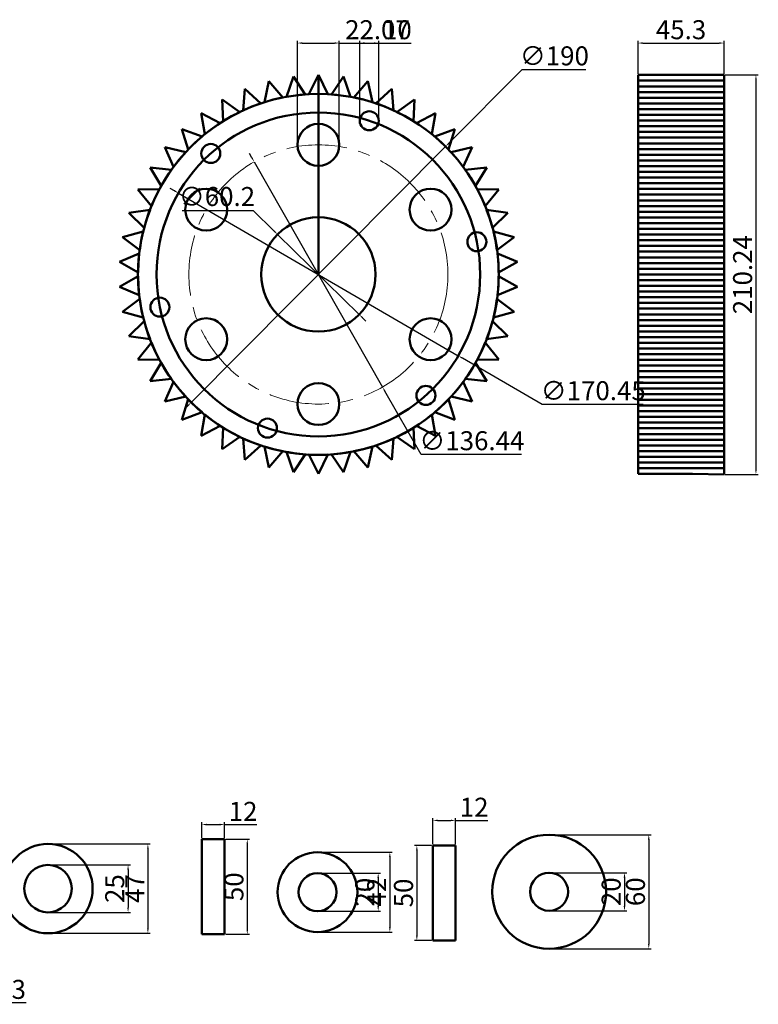
# Model space of a CAD drawing. Units: millimetres. Extents: x 828 to 2987, y 979 to 1807.
# Tile 4 of 6: x 1225 to 1614, y 1191 to 1709. Entities that reach past the tile are written whole.
import ezdxf

# ---------------------------------------------------------------- set-up
doc = ezdxf.new("R2010")
doc.units = ezdxf.units.MM
doc.linetypes.add('CENTER', pattern=[50.8, 31.75, -6.35, 6.35, -6.35])
for name, color, linetype, lineweight in [('M-CNTR', 1, 'CENTER', 18), ('M-DIMS', 2, 'Continuous', 25), ('M-OUTL', 7, 'Continuous', 50)]:
    doc.layers.add(name, color=color, linetype=linetype, lineweight=lineweight)
doc.styles.get("Standard").update_dxf_attribs({"font": 'arial.ttf'})
doc.dimstyles.new('ISO-25', dxfattribs={"dimtxt": 10, "dimasz": 2.5, "dimexe": 1.25, "dimexo": 0.625, "dimtad": 1, "dimtoh": 1, "dimdec": 0, "dimtxsty": 'Standard', "dimcen": 2.5, "dimadec": 0, "dimazin": 0, "dimtfac": 1, "dimtdec": 0, "dimtmove": 0, "dimatfit": 3, "dimfxl": 1, "dimarcsym": 0})

# ---------------------------------------------------------------- blocks, each defined once
blk = doc.blocks.new('*D29')
at = {"layer": 'Defpoints', "color": 0, "transparency": 16777216}
for p in [(1240.29, 1264.35), (1240.29, 1239.35), (1282.45, 1239.35)]:
    blk.add_point(p, dxfattribs=at)
at = {"layer": 'M-DIMS', "color": 0, "lineweight": -2, "transparency": 16777216}
for p, q in [((1240.91, 1264.35), (1283.7, 1264.35)), ((1282.45, 1261.85), (1282.45, 1241.85)), ((1240.91, 1239.35), (1283.7, 1239.35))]:
    blk.add_line(p, q, dxfattribs=at)
at = {"layer": 'M-DIMS', "color": 0, "transparency": 16777216}
for points in [[(1282.03, 1261.85), (1282.86, 1261.85), (1282.45, 1264.35)], [(1282.03, 1241.85), (1282.86, 1241.85), (1282.45, 1239.35)]]:
    blk.add_solid(points, dxfattribs=at)
at = {"layer": 'M-DIMS', "color": 0, "transparency": 16777216, "insert": (1276.72, 1251.85), "char_height": 10, "attachment_point": 5, "rotation": 90}
blk.add_mtext('25', dxfattribs=at)
blk = doc.blocks.new('*D30')
at = {"layer": 'Defpoints', "color": 0, "transparency": 16777216}
for p in [(1240.29, 1275.35), (1240.29, 1228.35), (1292.9, 1228.35)]:
    blk.add_point(p, dxfattribs=at)
at = {"layer": 'M-DIMS', "color": 0, "lineweight": -2, "transparency": 16777216}
for p, q in [((1240.91, 1275.35), (1294.15, 1275.35)), ((1292.9, 1272.85), (1292.9, 1230.85)), ((1240.91, 1228.35), (1294.15, 1228.35))]:
    blk.add_line(p, q, dxfattribs=at)
at = {"layer": 'M-DIMS', "color": 0, "transparency": 16777216}
for points in [[(1292.48, 1272.85), (1293.32, 1272.85), (1292.9, 1275.35)], [(1292.48, 1230.85), (1293.32, 1230.85), (1292.9, 1228.35)]]:
    blk.add_solid(points, dxfattribs=at)
at = {"layer": 'M-DIMS', "color": 0, "transparency": 16777216, "insert": (1287.28, 1251.85), "char_height": 10, "attachment_point": 5, "rotation": 90}
blk.add_mtext('47', dxfattribs=at)
blk = doc.blocks.new('*D31')
at = {"layer": 'Defpoints', "color": 0, "transparency": 16777216}
for p in [(1333.27, 1285.57), (1321.27, 1277.83), (1333.27, 1277.83)]:
    blk.add_point(p, dxfattribs=at)
at = {"layer": 'M-DIMS', "color": 0, "lineweight": -2, "transparency": 16777216}
for p, q in [((1321.27, 1278.45), (1321.27, 1286.82)), ((1323.77, 1285.57), (1330.77, 1285.57)), ((1333.27, 1278.45), (1333.27, 1286.82)), ((1333.27, 1285.57), (1350.3, 1285.57))]:
    blk.add_line(p, q, dxfattribs=at)
at = {"layer": 'M-DIMS', "color": 0, "transparency": 16777216}
for points in [[(1323.77, 1285.99), (1323.77, 1285.15), (1321.27, 1285.57)], [(1330.77, 1285.99), (1330.77, 1285.15), (1333.27, 1285.57)]]:
    blk.add_solid(points, dxfattribs=at)
at = {"layer": 'M-DIMS', "color": 0, "transparency": 16777216, "insert": (1343.03, 1291.22), "char_height": 10, "attachment_point": 5}
blk.add_mtext('12', dxfattribs=at)
blk = doc.blocks.new('*D32')
at = {"layer": 'Defpoints', "color": 0, "transparency": 16777216}
for p in [(1333.27, 1277.83), (1333.27, 1227.83), (1345.24, 1227.83)]:
    blk.add_point(p, dxfattribs=at)
at = {"layer": 'M-DIMS', "color": 0, "lineweight": -2, "transparency": 16777216}
for p, q in [((1333.89, 1277.83), (1346.49, 1277.83)), ((1345.24, 1275.33), (1345.24, 1230.33)), ((1333.89, 1227.83), (1346.49, 1227.83))]:
    blk.add_line(p, q, dxfattribs=at)
at = {"layer": 'M-DIMS', "color": 0, "transparency": 16777216}
for points in [[(1344.82, 1275.33), (1345.65, 1275.33), (1345.24, 1277.83)], [(1344.82, 1230.33), (1345.65, 1230.33), (1345.24, 1227.83)]]:
    blk.add_solid(points, dxfattribs=at)
at = {"layer": 'M-DIMS', "color": 0, "transparency": 16777216, "insert": (1339.5, 1252.83), "char_height": 10, "attachment_point": 5, "rotation": 90}
blk.add_mtext('50', dxfattribs=at)
blk = doc.blocks.new('*D33')
at = {"layer": 'Defpoints', "color": 0, "transparency": 16777216}
for p in [(1382.24, 1259.98), (1382.24, 1239.98), (1414.19, 1239.98)]:
    blk.add_point(p, dxfattribs=at)
at = {"layer": 'M-DIMS', "color": 0, "lineweight": -2, "transparency": 16777216}
for p, q in [((1382.86, 1259.98), (1415.44, 1259.98)), ((1414.19, 1257.48), (1414.19, 1242.48)), ((1382.86, 1239.98), (1415.44, 1239.98))]:
    blk.add_line(p, q, dxfattribs=at)
at = {"layer": 'M-DIMS', "color": 0, "transparency": 16777216}
for points in [[(1413.78, 1257.48), (1414.61, 1257.48), (1414.19, 1259.98)], [(1413.78, 1242.48), (1414.61, 1242.48), (1414.19, 1239.98)]]:
    blk.add_solid(points, dxfattribs=at)
at = {"layer": 'M-DIMS', "color": 0, "transparency": 16777216, "insert": (1408.46, 1249.98), "char_height": 10, "attachment_point": 5, "rotation": 90}
blk.add_mtext('20', dxfattribs=at)
blk = doc.blocks.new('*D34')
at = {"layer": 'Defpoints', "color": 0, "transparency": 16777216}
for p in [(1382.24, 1270.98), (1382.24, 1228.98), (1420.33, 1228.98)]:
    blk.add_point(p, dxfattribs=at)
at = {"layer": 'M-DIMS', "color": 0, "lineweight": -2, "transparency": 16777216}
for p, q in [((1382.86, 1270.98), (1421.58, 1270.98)), ((1420.33, 1268.48), (1420.33, 1231.48)), ((1382.86, 1228.98), (1421.58, 1228.98))]:
    blk.add_line(p, q, dxfattribs=at)
at = {"layer": 'M-DIMS', "color": 0, "transparency": 16777216}
for points in [[(1419.91, 1268.48), (1420.75, 1268.48), (1420.33, 1270.98)], [(1419.91, 1231.48), (1420.75, 1231.48), (1420.33, 1228.98)]]:
    blk.add_solid(points, dxfattribs=at)
at = {"layer": 'M-DIMS', "color": 0, "transparency": 16777216, "insert": (1414.68, 1249.98), "char_height": 10, "attachment_point": 5, "rotation": 90}
blk.add_mtext('42', dxfattribs=at)
blk = doc.blocks.new('*D35')
at = {"layer": 'Defpoints', "color": 0, "transparency": 16777216}
for p in [(1504.22, 1280.2), (1504.22, 1220.2), (1556.69, 1220.2)]:
    blk.add_point(p, dxfattribs=at)
at = {"layer": 'M-DIMS', "color": 0, "lineweight": -2, "transparency": 16777216}
for p, q in [((1504.85, 1280.2), (1557.94, 1280.2)), ((1556.69, 1277.7), (1556.69, 1222.7)), ((1504.85, 1220.2), (1557.94, 1220.2))]:
    blk.add_line(p, q, dxfattribs=at)
at = {"layer": 'M-DIMS', "color": 0, "transparency": 16777216}
for points in [[(1556.27, 1277.7), (1557.11, 1277.7), (1556.69, 1280.2)], [(1556.27, 1222.7), (1557.11, 1222.7), (1556.69, 1220.2)]]:
    blk.add_solid(points, dxfattribs=at)
at = {"layer": 'M-DIMS', "color": 0, "transparency": 16777216, "insert": (1550.96, 1250.2), "char_height": 10, "attachment_point": 5, "rotation": 90}
blk.add_mtext('60', dxfattribs=at)
blk = doc.blocks.new('*D36')
at = {"layer": 'Defpoints', "color": 0, "transparency": 16777216}
for p in [(1504.22, 1260.2), (1504.22, 1240.2), (1543.9, 1240.2)]:
    blk.add_point(p, dxfattribs=at)
at = {"layer": 'M-DIMS', "color": 0, "lineweight": -2, "transparency": 16777216}
for p, q in [((1504.85, 1260.2), (1545.15, 1260.2)), ((1543.9, 1257.7), (1543.9, 1242.7)), ((1504.85, 1240.2), (1545.15, 1240.2))]:
    blk.add_line(p, q, dxfattribs=at)
at = {"layer": 'M-DIMS', "color": 0, "transparency": 16777216}
for points in [[(1543.48, 1257.7), (1544.32, 1257.7), (1543.9, 1260.2)], [(1543.48, 1242.7), (1544.32, 1242.7), (1543.9, 1240.2)]]:
    blk.add_solid(points, dxfattribs=at)
at = {"layer": 'M-DIMS', "color": 0, "transparency": 16777216, "insert": (1538.17, 1250.2), "char_height": 10, "attachment_point": 5, "rotation": 90}
blk.add_mtext('20', dxfattribs=at)
blk = doc.blocks.new('*D37')
at = {"layer": 'Defpoints', "color": 0, "transparency": 16777216}
for p in [(1454.95, 1287.75), (1442.95, 1274.56), (1454.95, 1274.56)]:
    blk.add_point(p, dxfattribs=at)
at = {"layer": 'M-DIMS', "color": 0, "lineweight": -2, "transparency": 16777216}
for p, q in [((1442.95, 1275.18), (1442.95, 1289)), ((1445.45, 1287.75), (1452.45, 1287.75)), ((1454.95, 1275.18), (1454.95, 1289)), ((1454.95, 1287.75), (1471.98, 1287.75))]:
    blk.add_line(p, q, dxfattribs=at)
at = {"layer": 'M-DIMS', "color": 0, "transparency": 16777216}
for points in [[(1445.45, 1288.17), (1445.45, 1287.34), (1442.95, 1287.75)], [(1452.45, 1288.17), (1452.45, 1287.34), (1454.95, 1287.75)]]:
    blk.add_solid(points, dxfattribs=at)
at = {"layer": 'M-DIMS', "color": 0, "transparency": 16777216, "insert": (1464.71, 1293.4), "char_height": 10, "attachment_point": 5}
blk.add_mtext('12', dxfattribs=at)
blk = doc.blocks.new('*D38')
at = {"layer": 'Defpoints', "color": 0, "transparency": 16777216}
for p in [(1442.95, 1274.56), (1434.54, 1224.56), (1442.95, 1224.56)]:
    blk.add_point(p, dxfattribs=at)
at = {"layer": 'M-DIMS', "color": 0, "lineweight": -2, "transparency": 16777216}
for p, q in [((1442.32, 1274.56), (1433.29, 1274.56)), ((1434.54, 1272.06), (1434.54, 1227.06)), ((1442.32, 1224.56), (1433.29, 1224.56))]:
    blk.add_line(p, q, dxfattribs=at)
at = {"layer": 'M-DIMS', "color": 0, "transparency": 16777216}
for points in [[(1434.13, 1272.06), (1434.96, 1272.06), (1434.54, 1274.56)], [(1434.13, 1227.06), (1434.96, 1227.06), (1434.54, 1224.56)]]:
    blk.add_solid(points, dxfattribs=at)
at = {"layer": 'M-DIMS', "color": 0, "transparency": 16777216, "insert": (1428.81, 1249.56), "char_height": 10, "attachment_point": 5, "rotation": 90}
blk.add_mtext('50', dxfattribs=at)
blk = doc.blocks.new('*U39')
for p, q in [((-5, -5.09), (0, 5.09)), ((5, -5.09), (0, 5.09)), ((0, -4.91), (-5, -5.09)), ((0, -4.91), (5, -5.09))]:
    blk.add_line(p, q)
blk = doc.blocks.new('*U40')
at = {"layer": 'M-OUTL', "color": 0, "linetype": 'ByBlock', "lineweight": -2, "transparency": 16777216}
for p, rotation in [((1370.16, 1674.27), 7.199999999999979), ((1395.21, 1674.27), 352.8000000000002), ((1345.91, 1668.04), 21.60000000000001), ((1357.84, 1671.92), 14.40000000000001), ((1407.53, 1671.92), 345.6000000000001), ((1419.46, 1668.04), 338.4), ((1334.55, 1662.7), 28.79999999999999), ((1430.82, 1662.7), 331.2000000000001), ((1323.96, 1655.98), 35.99999999999999), ((1441.41, 1655.98), 324), ((1314.29, 1647.98), 43.20000000000002), ((1451.08, 1647.98), 316.8), ((1305.7, 1638.83), 50.4), ((1459.67, 1638.83), 309.6000000000001), ((1298.33, 1628.68), 57.6), ((1467.04, 1628.68), 302.4000000000001), ((1292.28, 1617.69), 64.80000000000001), ((1473.09, 1617.69), 295.2), ((1287.67, 1606.02), 72), ((1477.7, 1606.02), 288), ((1284.55, 1593.87), 79.2), ((1480.82, 1593.87), 280.8), ((1282.97, 1581.42), 86.40000000000002), ((1482.4, 1581.42), 273.6), ((1282.97, 1568.87), 93.60000000000001), ((1482.4, 1568.87), 266.4000000000001), ((1284.55, 1556.43), 100.8), ((1480.82, 1556.43), 259.2), ((1287.67, 1544.27), 108), ((1477.7, 1544.27), 252), ((1292.28, 1532.61), 115.2), ((1473.09, 1532.61), 244.8), ((1298.33, 1521.61), 122.4), ((1467.04, 1521.61), 237.6), ((1305.7, 1511.46), 129.6), ((1459.67, 1511.46), 230.4), ((1314.29, 1502.32), 136.8), ((1451.08, 1502.32), 223.2), ((1323.96, 1494.32), 144), ((1441.41, 1494.32), 216), ((1334.55, 1487.6), 151.2), ((1430.82, 1487.6), 208.8), ((1345.91, 1482.26), 158.4), ((1419.46, 1482.26), 201.6), ((1357.84, 1478.38), 165.6), ((1407.53, 1478.38), 194.4), ((1370.16, 1476.03), 172.8000000000001), ((1382.69, 1475.24), 180), ((1395.21, 1476.03), 187.1999999999999)]:
    blk.add_blockref('*U39', p, dxfattribs=dict(at, rotation=rotation))
blk.add_blockref('*U39', (1382.69, 1675.06), dxfattribs=at)
blk = doc.blocks.new('*U41')
blk.add_circle((0, 0), 11.03)
blk = doc.blocks.new('*U42')
at = {"layer": 'M-OUTL', "color": 0, "linetype": 'ByBlock', "lineweight": -2, "transparency": 16777216}
blk.add_blockref('*U41', (1382.69, 1643.37), dxfattribs=at)
for p, rotation in [((1323.6, 1609.26), 60), ((1441.77, 1609.26), 300), ((1323.6, 1541.04), 120), ((1441.77, 1541.04), 240), ((1382.69, 1506.93), 180)]:
    blk.add_blockref('*U41', p, dxfattribs=dict(at, rotation=rotation))
blk = doc.blocks.new('*U43')
blk.add_circle((0, 0), 5)
blk = doc.blocks.new('*U44')
at = {"layer": 'M-OUTL', "color": 0, "linetype": 'ByBlock', "lineweight": -2, "transparency": 16777216}
blk.add_blockref('*U43', (1409.5, 1656.04), dxfattribs=at)
for p, rotation in [((1326.04, 1638.82), 60), ((1466.15, 1592.37), 300), ((1299.22, 1557.93), 120), ((1439.33, 1511.48), 240), ((1355.87, 1494.26), 180)]:
    blk.add_blockref('*U43', p, dxfattribs=dict(at, rotation=rotation))
blk = doc.blocks.new('*D94')
at = {"layer": 'Defpoints', "color": 0, "transparency": 16777216}
for p in [(1393.72, 1696.95), (1371.65, 1643.37), (1393.72, 1643.37)]:
    blk.add_point(p, dxfattribs=at)
at = {"layer": 'M-DIMS', "color": 0, "lineweight": -2, "transparency": 16777216}
for p, q in [((1371.65, 1644), (1371.65, 1698.2)), ((1374.15, 1696.95), (1391.22, 1696.95)), ((1393.72, 1644), (1393.72, 1698.2)), ((1393.72, 1696.95), (1431.39, 1696.95))]:
    blk.add_line(p, q, dxfattribs=at)
at = {"layer": 'M-DIMS', "color": 0, "transparency": 16777216}
for points in [[(1374.15, 1697.36), (1374.15, 1696.53), (1371.65, 1696.95)], [(1391.22, 1697.36), (1391.22, 1696.53), (1393.72, 1696.95)]]:
    blk.add_solid(points, dxfattribs=at)
at = {"layer": 'M-DIMS', "color": 0, "transparency": 16777216, "insert": (1413.8, 1702.68), "char_height": 10, "attachment_point": 5}
blk.add_mtext('22.07', dxfattribs=at)
blk = doc.blocks.new('*D95')
at = {"layer": 'Defpoints', "color": 0, "transparency": 16777216}
for p in [(1414.5, 1696.95), (1404.5, 1656.04), (1414.5, 1656.04)]:
    blk.add_point(p, dxfattribs=at)
at = {"layer": 'M-DIMS', "color": 0, "lineweight": -2, "transparency": 16777216}
for p, q in [((1404.5, 1656.67), (1404.5, 1698.2)), ((1407, 1696.95), (1412, 1696.95)), ((1414.5, 1656.67), (1414.5, 1698.2)), ((1414.5, 1696.95), (1431.6, 1696.95))]:
    blk.add_line(p, q, dxfattribs=at)
at = {"layer": 'M-DIMS', "color": 0, "transparency": 16777216}
for points in [[(1407, 1697.36), (1407, 1696.53), (1404.5, 1696.95)], [(1412, 1697.36), (1412, 1696.53), (1414.5, 1696.95)]]:
    blk.add_solid(points, dxfattribs=at)
at = {"layer": 'M-DIMS', "color": 0, "transparency": 16777216, "insert": (1424.3, 1702.68), "char_height": 10, "attachment_point": 5}
blk.add_mtext('10', dxfattribs=at)
blk = doc.blocks.new('*D96')
at = {"layer": 'Defpoints', "color": 0, "transparency": 16777216}
for p in [(1596.33, 1696.95), (1551.03, 1680.15), (1596.33, 1680.15)]:
    blk.add_point(p, dxfattribs=at)
at = {"layer": 'M-DIMS', "color": 0, "lineweight": -2, "transparency": 16777216}
for p, q in [((1551.03, 1680.77), (1551.03, 1698.2)), ((1553.53, 1696.95), (1593.83, 1696.95)), ((1596.33, 1680.77), (1596.33, 1698.2))]:
    blk.add_line(p, q, dxfattribs=at)
at = {"layer": 'M-DIMS', "color": 0, "transparency": 16777216}
for points in [[(1553.53, 1697.36), (1553.53, 1696.53), (1551.03, 1696.95)], [(1593.83, 1697.36), (1593.83, 1696.53), (1596.33, 1696.95)]]:
    blk.add_solid(points, dxfattribs=at)
at = {"layer": 'M-DIMS', "color": 0, "transparency": 16777216, "insert": (1573.68, 1702.68), "char_height": 10, "attachment_point": 5}
blk.add_mtext('45.3', dxfattribs=at)
blk = doc.blocks.new('*D97')
at = {"layer": 'Defpoints', "color": 0, "transparency": 16777216}
for p in [(1596.33, 1680.15), (1596.33, 1469.91), (1613.13, 1469.91)]:
    blk.add_point(p, dxfattribs=at)
at = {"layer": 'M-DIMS', "color": 0, "lineweight": -2, "transparency": 16777216}
for p, q in [((1596.96, 1680.15), (1614.38, 1680.15)), ((1613.13, 1677.65), (1613.13, 1472.41)), ((1596.96, 1469.91), (1614.38, 1469.91))]:
    blk.add_line(p, q, dxfattribs=at)
at = {"layer": 'M-DIMS', "color": 0, "transparency": 16777216}
for points in [[(1612.72, 1677.65), (1613.55, 1677.65), (1613.13, 1680.15)], [(1612.72, 1472.41), (1613.55, 1472.41), (1613.13, 1469.91)]]:
    blk.add_solid(points, dxfattribs=at)
at = {"layer": 'M-DIMS', "color": 0, "transparency": 16777216, "insert": (1607.4, 1575.03), "char_height": 10, "attachment_point": 5, "rotation": 90}
blk.add_mtext('210.24', dxfattribs=at)
blk = doc.blocks.new('*D128')
at = {"layer": 'Defpoints', "color": 0, "transparency": 16777216}
for p in [(1105.21, 1219.26), (1159.88, 1202.09)]:
    blk.add_point(p, dxfattribs=at)
at = {"layer": 'M-DIMS', "color": 0, "lineweight": -2, "transparency": 16777216}
for p, q in [((1105.21, 1219.26), (1159.88, 1202.09)), ((1192.68, 1191.78), (1162.27, 1201.34)), ((1228.86, 1191.78), (1192.68, 1191.78))]:
    blk.add_line(p, q, dxfattribs=at)
at = {"layer": 'M-DIMS', "color": 0, "transparency": 16777216}
blk.add_solid([(1162.39, 1201.73), (1162.14, 1200.94), (1159.88, 1202.09)], dxfattribs=at)
at = {"layer": 'M-DIMS', "color": 0, "transparency": 16777216, "insert": (1211.08, 1197.51), "char_height": 10, "attachment_point": 5}
blk.add_mtext('R57.3', dxfattribs=at)
blk = doc.blocks.new('*D135')
at = {"layer": 'Defpoints', "color": 0, "transparency": 16777216}
for p in [(1449.69, 1642.49), (1315.68, 1507.8)]:
    blk.add_point(p, dxfattribs=at)
at = {"layer": 'M-DIMS', "color": 0, "lineweight": -2, "transparency": 16777216}
for p, q in [((1489.89, 1682.9), (1451.45, 1644.26)), ((1523.46, 1682.9), (1489.89, 1682.9)), ((1315.68, 1507.8), (1449.69, 1642.49)), ((1313.92, 1506.03), (1312.15, 1504.26))]:
    blk.add_line(p, q, dxfattribs=at)
at = {"layer": 'M-DIMS', "color": 0, "transparency": 16777216}
for points in [[(1451.16, 1644.56), (1451.75, 1643.97), (1449.69, 1642.49)], [(1313.62, 1506.33), (1314.21, 1505.74), (1315.68, 1507.8)]]:
    blk.add_solid(points, dxfattribs=at)
at = {"layer": 'M-DIMS', "color": 0, "transparency": 16777216, "insert": (1506.99, 1688.91), "char_height": 10, "attachment_point": 5}
blk.add_mtext('∅190', dxfattribs=at)
blk = doc.blocks.new('*D136')
at = {"layer": 'Defpoints', "color": 0, "transparency": 16777216}
for p in [(1308.99, 1617.96), (1456.38, 1532.34)]:
    blk.add_point(p, dxfattribs=at)
at = {"layer": 'M-DIMS', "color": 0, "lineweight": -2, "transparency": 16777216}
for p, q in [((1306.83, 1619.21), (1304.67, 1620.47)), ((1308.99, 1617.96), (1456.38, 1532.34)), ((1500.59, 1506.65), (1458.54, 1531.08)), ((1553.68, 1506.65), (1500.59, 1506.65))]:
    blk.add_line(p, q, dxfattribs=at)
at = {"layer": 'M-DIMS', "color": 0, "transparency": 16777216}
for points in [[(1307.04, 1619.57), (1306.62, 1618.85), (1308.99, 1617.96)], [(1458.75, 1531.44), (1458.33, 1530.72), (1456.38, 1532.34)]]:
    blk.add_solid(points, dxfattribs=at)
at = {"layer": 'M-DIMS', "color": 0, "transparency": 16777216, "insert": (1527.45, 1512.67), "char_height": 10, "attachment_point": 5}
blk.add_mtext('∅170.45', dxfattribs=at)
blk = doc.blocks.new('*D137')
at = {"layer": 'Defpoints', "color": 0, "transparency": 16777216}
for p in [(1348.9, 1634.42), (1416.47, 1515.88)]:
    blk.add_point(p, dxfattribs=at)
at = {"layer": 'M-DIMS', "color": 0, "lineweight": -2, "transparency": 16777216}
for p, q in [((1347.66, 1636.59), (1346.42, 1638.76)), ((1348.9, 1634.42), (1416.47, 1515.88)), ((1436.74, 1480.32), (1417.71, 1513.71)), ((1489.72, 1480.32), (1436.74, 1480.32))]:
    blk.add_line(p, q, dxfattribs=at)
at = {"layer": 'M-DIMS', "color": 0, "transparency": 16777216}
for points in [[(1348.02, 1636.8), (1347.3, 1636.38), (1348.9, 1634.42)], [(1418.07, 1513.91), (1417.35, 1513.5), (1416.47, 1515.88)]]:
    blk.add_solid(points, dxfattribs=at)
at = {"layer": 'M-DIMS', "color": 0, "transparency": 16777216, "insert": (1463.54, 1486.33), "char_height": 10, "attachment_point": 5}
blk.add_mtext('∅136.44', dxfattribs=at)
blk = doc.blocks.new('*D138')
at = {"layer": 'Defpoints', "color": 0, "transparency": 16777216}
for p in [(1361.19, 1596.22), (1404.18, 1554.08)]:
    blk.add_point(p, dxfattribs=at)
at = {"layer": 'M-DIMS', "color": 0, "lineweight": -2, "transparency": 16777216}
for p, q in [((1310.91, 1608.86), (1348.29, 1608.86)), ((1348.29, 1608.86), (1359.4, 1597.97)), ((1404.18, 1554.08), (1361.19, 1596.22)), ((1405.97, 1552.33), (1407.76, 1550.58))]:
    blk.add_line(p, q, dxfattribs=at)
at = {"layer": 'M-DIMS', "color": 0, "transparency": 16777216}
for points in [[(1359.69, 1598.27), (1359.11, 1597.67), (1361.19, 1596.22)], [(1406.26, 1552.63), (1405.68, 1552.03), (1404.18, 1554.08)]]:
    blk.add_solid(points, dxfattribs=at)
at = {"layer": 'M-DIMS', "color": 0, "transparency": 16777216, "insert": (1329.28, 1614.87), "char_height": 10, "attachment_point": 5}
blk.add_mtext('∅60.2', dxfattribs=at)

msp = doc.modelspace()

# ---------------------------------------------------------------- linework, layer by layer
at = {"layer": 'M-CNTR'}
msp.add_circle((1382.685, 1575.1483), 68.2219, dxfattribs=at)
at = {"layer": 'M-OUTL'}
for p, q in [((1382.685, 1575.1483), (1382.685, 1680.1483)), ((1551.0317, 1680.1483), (1596.3344, 1680.1483)), ((1551.0317, 1670.4944), (1551.0317, 1680.1483)), ((1551.0317, 1680.1483), (1551.0317, 1677.1483)), ((1596.3344, 1680.1483), (1596.3344, 1469.9065)), ((1551.0317, 1677.1483), (1596.3344, 1677.1483)), ((1596.3344, 1674.1483), (1551.0317, 1674.1483)), ((1382.685, 1670.1483), (1382.685, 1670.1483)), ((1551.0317, 1671.1483), (1596.3344, 1671.1483)), ((1551.0317, 1670.4944), (1551.0317, 1470.1483)), ((1409.5992, 1666.1901), (1409.5998, 1666.2559)), ((1596.3344, 1668.1483), (1551.0317, 1668.1483)), ((1551.0317, 1665.1483), (1596.3344, 1665.1483)), ((1596.3344, 1662.1483), (1551.0317, 1662.1483)), ((1551.0317, 1659.1483), (1596.3344, 1659.1483)), ((1596.3344, 1656.1483), (1551.0317, 1656.1483)), ((1551.0317, 1653.1483), (1596.3344, 1653.1483)), ((1596.3344, 1650.1483), (1551.0317, 1650.1483)), ((1551.0317, 1647.1483), (1596.3344, 1647.1483)), ((1596.3344, 1644.1483), (1551.0317, 1644.1483)), ((1551.0317, 1641.1483), (1596.3344, 1641.1483)), ((1596.3344, 1638.1483), (1551.0317, 1638.1483)), ((1551.0317, 1635.1483), (1596.3344, 1635.1483)), ((1596.3344, 1632.1483), (1551.0317, 1632.1483)), ((1551.0317, 1629.1483), (1596.3344, 1629.1483)), ((1596.3344, 1626.1483), (1551.0317, 1626.1483)), ((1551.0317, 1623.1483), (1596.3344, 1623.1483)), ((1596.3344, 1620.1483), (1551.0317, 1620.1483)), ((1551.0317, 1617.1483), (1596.3344, 1617.1483)), ((1596.3344, 1614.1483), (1551.0317, 1614.1483)), ((1551.0317, 1611.1483), (1596.3344, 1611.1483)), ((1596.3344, 1608.1483), (1551.0317, 1608.1483)), ((1551.0317, 1605.1483), (1596.3344, 1605.1483)), ((1596.3344, 1602.1483), (1551.0317, 1602.1483)), ((1551.0317, 1599.1483), (1596.3344, 1599.1483)), ((1596.3344, 1596.1483), (1551.0317, 1596.1483)), ((1551.0317, 1593.1483), (1596.3344, 1593.1483)), ((1596.3344, 1590.1483), (1551.0317, 1590.1483)), ((1551.0317, 1587.1483), (1596.3344, 1587.1483)), ((1596.3344, 1584.1483), (1551.0317, 1584.1483)), ((1551.0317, 1581.1483), (1596.3344, 1581.1483)), ((1596.3344, 1578.1483), (1551.0317, 1578.1483)), ((1551.0317, 1575.1483), (1596.3344, 1575.1483)), ((1596.3344, 1572.1483), (1551.0317, 1572.1483)), ((1551.0317, 1569.1483), (1596.3344, 1569.1483)), ((1596.3344, 1566.1483), (1551.0317, 1566.1483)), ((1551.0317, 1563.1483), (1596.3344, 1563.1483)), ((1596.3344, 1560.1483), (1551.0317, 1560.1483)), ((1551.0317, 1557.1483), (1596.3344, 1557.1483)), ((1596.3344, 1554.1483), (1551.0317, 1554.1483)), ((1551.0317, 1551.1483), (1596.3344, 1551.1483)), ((1596.3344, 1548.1483), (1551.0317, 1548.1483)), ((1551.0317, 1545.1483), (1596.3344, 1545.1483)), ((1596.3344, 1542.1483), (1551.0317, 1542.1483)), ((1551.0317, 1539.1483), (1596.3344, 1539.1483)), ((1596.3344, 1536.1483), (1551.0317, 1536.1483)), ((1551.0317, 1533.1483), (1596.3344, 1533.1483)), ((1596.3344, 1530.1483), (1551.0317, 1530.1483)), ((1551.0317, 1527.1483), (1596.3344, 1527.1483)), ((1596.3344, 1524.1483), (1551.0317, 1524.1483)), ((1551.0317, 1521.1483), (1596.3344, 1521.1483)), ((1596.3344, 1518.1483), (1551.0317, 1518.1483)), ((1551.0317, 1515.1483), (1596.3344, 1515.1483)), ((1596.3344, 1512.1483), (1551.0317, 1512.1483)), ((1551.0317, 1509.1483), (1596.3344, 1509.1483)), ((1596.3344, 1506.1483), (1551.0317, 1506.1483)), ((1551.0317, 1503.1483), (1596.3344, 1503.1483)), ((1596.3344, 1500.1483), (1551.0317, 1500.1483)), ((1551.0317, 1497.1483), (1596.3344, 1497.1483)), ((1596.3344, 1494.1483), (1551.0317, 1494.1483)), ((1551.0317, 1491.1483), (1596.3344, 1491.1483)), ((1596.3344, 1488.1483), (1551.0317, 1488.1483)), ((1551.0317, 1485.1483), (1596.3344, 1485.1483)), ((1596.3344, 1482.1483), (1551.0317, 1482.1483)), ((1551.0317, 1479.1483), (1596.3344, 1479.1483)), ((1596.3344, 1476.1483), (1551.0317, 1476.1483)), ((1551.0317, 1473.1483), (1596.3344, 1473.1483)), ((1551.0317, 1470.1483), (1579.805, 1470.1483)), ((1596.3344, 1469.9065), (1579.805, 1470.1483)), ((1321.2663, 1277.8286), (1321.2663, 1227.8286)), ((1333.2663, 1277.8286), (1321.2663, 1277.8286)), ((1333.2663, 1227.8286), (1333.2663, 1277.8286)), ((1442.9478, 1274.5568), (1442.9478, 1224.5568)), ((1454.9478, 1274.5568), (1442.9478, 1274.5568)), ((1454.9478, 1224.5568), (1454.9478, 1274.5568)), ((1321.2663, 1227.8286), (1333.2663, 1227.8286)), ((1442.9478, 1224.5568), (1454.9478, 1224.5568))]:
    msp.add_line(p, q, dxfattribs=at)
for centre, radius in [((1382.685, 1575.1483), 95), ((1382.685, 1575.1483), 85.2226), ((1382.685, 1575.1483), 30.1021), ((1504.221, 1250.2042), 30), ((1240.2869, 1251.8522), 23.5), ((1382.2371, 1249.9809), 21), ((1240.2869, 1251.8522), 12.5), ((1382.2371, 1249.9809), 10), ((1504.221, 1250.2042), 10)]:
    msp.add_circle(centre, radius, dxfattribs=at)

# ---------------------------------------------------------------- block references
for name in ['*U40', '*U44', '*U42']:
    msp.add_blockref(name, (0, 0), dxfattribs=at)

# ---------------------------------------------------------------- dimensions: what is measured, and where the dimension line sits
at = {"layer": 'M-DIMS'}
for base, p1, p2, override, picture, middle in [((1393.7197, 1696.9483), (1371.6503, 1643.3702), (1393.7197, 1643.3702), {"dimdec": 2, "dimlfac": 1, "dimrnd": 0, "dimzin": 0, "dimdsep": 46, "dimlunit": 2}, '*D94', (1413.8024, 1702.679)), ((1414.5043, 1696.9483), (1404.5043, 1656.0409), (1414.5043, 1656.0409), {"dimdec": 0, "dimlfac": 1, "dimrnd": 0, "dimzin": 0, "dimdsep": 46, "dimlunit": 2}, '*D95', (1424.3039, 1702.679)), ((1596.3344, 1696.9483), (1551.0317, 1680.1483), (1596.3344, 1680.1483), {"dimdec": 1, "dimlfac": 1, "dimrnd": 0, "dimzin": 0, "dimdsep": 46, "dimlunit": 2}, '*D96', (1573.683, 1702.6824)), ((1333.2663, 1285.571), (1321.2663, 1277.8286), (1333.2663, 1277.8286), {"dimclrd": 0, "dimclre": 0, "dimclrt": 0}, '*D31', (1343.0318, 1291.2165)), ((1454.9478, 1287.7536), (1442.9478, 1274.5568), (1454.9478, 1274.5568), {"dimclrd": 0, "dimclre": 0, "dimclrt": 0}, '*D37', (1464.7133, 1293.3991))]:
    dim = msp.add_linear_dim(base=base, p1=p1, p2=p2, dimstyle='ISO-25', override=override, dxfattribs=at)
    dim.commit()
    dim.dimension.update_dxf_attribs({"geometry": picture, "text_midpoint": middle})
for p1, p2, override, picture, middle in [((1315.6789, 1507.8045), (1449.6911, 1642.4921), {"dimdec": 0, "dimlfac": 1, "dimrnd": 0, "dimzin": 0, "dimdsep": 46, "dimlunit": 2}, '*D135', (1506.9898, 1682.8983)), ((1348.901, 1634.4177), (1416.469, 1515.8789), {"dimdec": 2, "dimlfac": 1, "dimrnd": 0, "dimzin": 0, "dimdsep": 46, "dimlunit": 2}, '*D137', (1463.5411, 1480.3173)), ((1308.9943, 1617.9568), (1456.3757, 1532.3398), {"dimdec": 2, "dimlfac": 1, "dimrnd": 0, "dimzin": 0, "dimdsep": 46, "dimlunit": 2}, '*D136', (1527.4498, 1506.6547)), ((1404.1841, 1554.0788), (1361.1859, 1596.2178), {"dimdec": 1, "dimlfac": 1, "dimrnd": 0, "dimzin": 0, "dimdsep": 46, "dimlunit": 2}, '*D138', (1329.2849, 1608.8595))]:
    dim = msp.add_diameter_dim_2p(p1=p1, p2=p2, dimstyle='ISO-25', override=override, dxfattribs=at)
    dim.commit()
    dim.dimension.update_dxf_attribs({"geometry": picture, "text_midpoint": middle, "dimtype": 163})
for base, p1, p2, override, picture, middle in [((1613.1344, 1469.9065), (1596.3344, 1680.1483), (1596.3344, 1469.9065), {"dimdec": 2, "dimlfac": 1, "dimrnd": 0, "dimzin": 0, "dimdsep": 46, "dimlunit": 2}, '*D97', (1607.4036, 1575.0274)), ((1556.6907, 1220.2042), (1504.221, 1280.2042), (1504.221, 1220.2042), {"dimclrd": 0, "dimclre": 0, "dimclrt": 0}, '*D35', (1550.96, 1250.2042)), ((1292.9011, 1228.3522), (1240.2869, 1275.3522), (1240.2869, 1228.3522), {"dimclrd": 0, "dimclre": 0, "dimclrt": 0}, '*D30', (1287.2761, 1251.8522)), ((1345.235, 1227.8286), (1333.2663, 1277.8286), (1333.2663, 1227.8286), {"dimclrd": 0, "dimclre": 0, "dimclrt": 0}, '*D32', (1339.5043, 1252.8286)), ((1420.3288, 1228.9809), (1382.2371, 1270.9809), (1382.2371, 1228.9809), {"dimclrd": 0, "dimclre": 0, "dimclrt": 0}, '*D34', (1414.6834, 1249.9809)), ((1434.5442, 1224.5568), (1442.9478, 1274.5568), (1442.9478, 1224.5568), {"dimclrd": 0, "dimclre": 0, "dimclrt": 0}, '*D38', (1428.8135, 1249.5568)), ((1282.4457, 1239.3522), (1240.2869, 1264.3522), (1240.2869, 1239.3522), {"dimclrd": 0, "dimclre": 0, "dimclrt": 0}, '*D29', (1276.715, 1251.8522)), ((1414.1918, 1239.9809), (1382.2371, 1259.9809), (1382.2371, 1239.9809), {"dimclrd": 0, "dimclre": 0, "dimclrt": 0}, '*D33', (1408.4611, 1249.9809)), ((1543.8987, 1240.2042), (1504.221, 1260.2042), (1504.221, 1240.2042), {"dimclrd": 0, "dimclre": 0, "dimclrt": 0}, '*D36', (1538.168, 1250.2042))]:
    dim = msp.add_linear_dim(base=base, p1=p1, p2=p2, angle=90, dimstyle='ISO-25', override=override, dxfattribs=at)
    dim.commit()
    dim.dimension.update_dxf_attribs({"geometry": picture, "text_midpoint": middle})
dim = msp.add_radius_dim(center=(1105.2149, 1219.2594), mpoint=(1159.8837, 1202.0851), dimstyle='ISO-25', override={"dimdec": 1, "dimlfac": 1, "dimrnd": 0, "dimzin": 0, "dimdsep": 46, "dimlunit": 2}, dxfattribs=at)
dim.commit()
dim.dimension.update_dxf_attribs({"geometry": '*D128', "text_midpoint": (1211.0828, 1191.7805), "dimtype": 164})

doc.saveas('drawing.dxf')
